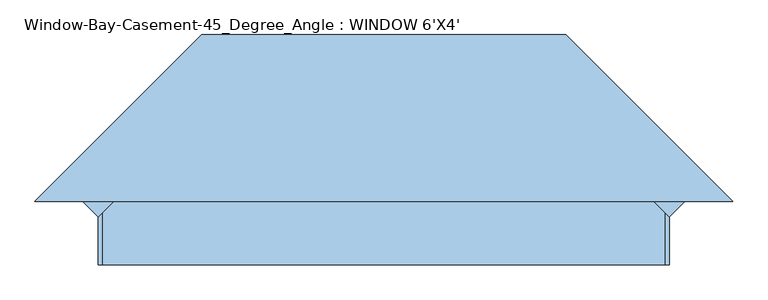
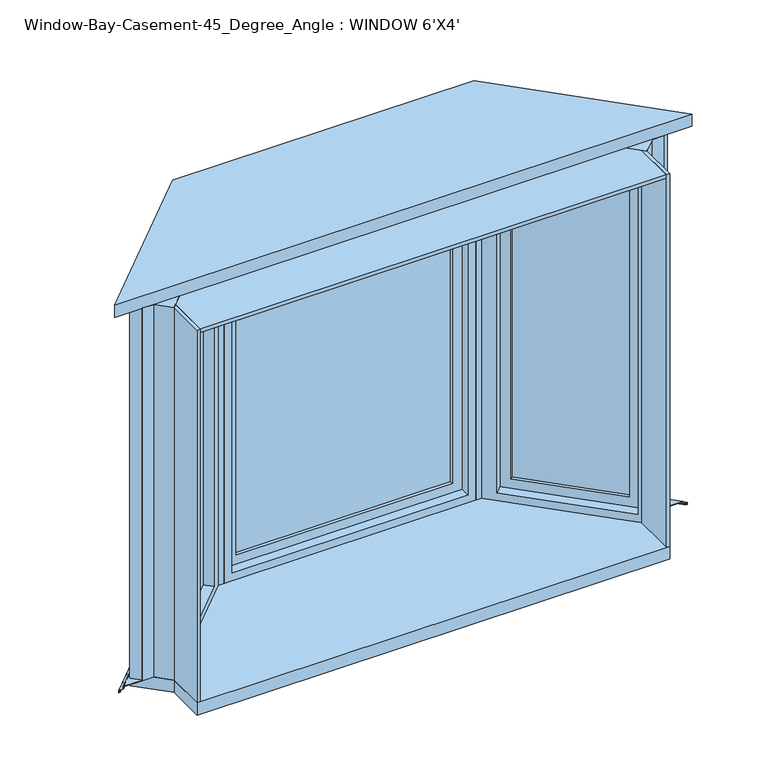
"""IFC4 building model written with IfcOpenShell, lengths in millimetres: window geometry, Window-Bay-Casement-45_Degree_Angle : WINDOW 6'X4'."""

from ifc_helpers import new_model, si_unit, frame, origin, place, context, project, spatial, polyline, outline, extrude, faceted_brep, source, transform, mapped, element, save


def window_bay_casement_45_degree_angle_window_6_x4_737bffb6(model_context):
    return source(origin(), model_context, "Body", "SolidModel", [
        extrude(outline(polyline([(914.4, 150.9914087), (909.9098719, 146.5012806), (619.1637138, 437.2474388), (623.6538418, 441.7375668), (914.4, 150.9914087)])), frame((0.0, 0.0, 730.25), z_axis=(0.0, 0.0, 1.0), x_axis=(1.0, 0.0, 0.0)), (0.0, 0.0, 1.0), 1384.3),
        extrude(outline(polyline([(905.4197439, 142.0111525), (900.9296158, 137.5210245), (610.1834576, 428.2671827), (614.6735857, 432.7573107), (905.4197439, 142.0111525)])), frame((0.0, 0.0, 730.25), z_axis=(0.0, 0.0, 1.0), x_axis=(1.0, 0.0, 0.0)), (0.0, 0.0, 1.0), 1384.3),
        extrude(outline(polyline([(1441.45, 57.15), (1441.45, -468.3271601), (-57.15, -468.3271601), (-57.15, 57.15), (1441.45, 57.15)]), holes=[polyline([(1384.3, -411.1771601), (1384.3, 0.0), (0.0, 0.0), (0.0, -411.1771601), (1384.3, -411.1771601)])]), frame((891.9493597, 128.5407684, 730.25), z_axis=(0.7071067811865468, 0.7071067811865483, 0.0), x_axis=(0.0, 0.0, 1.0)), (0.0, 0.0, 1.0), 44.45),
        faceted_brep([(509.4085913, 457.2, 2184.4), (914.4, 52.2085913, 2184.4), (963.7914087, 101.6, 2184.4), (1008.6926893, 101.6, 2184.4), (551.4926893, 558.8, 2184.4), (932.3605122, 88.1296158, 2171.7), (560.792049, 459.6980791, 2171.7), (605.6933296, 504.5993597, 2171.7), (977.2617928, 133.0308964, 2171.7), (891.9493597, 74.6592316, 2152.65), (547.3216648, 419.2869265, 2152.65), (574.2624332, 446.2276949, 2152.65), (918.8901281, 101.6, 2152.65), (560.792049, 459.6980791, 673.1), (605.6933296, 504.5993597, 673.1), (547.3216648, 419.2869265, 692.15), (574.2624332, 446.2276949, 692.15), (551.4926893, 558.8, 660.4), (1008.6926893, 101.6, 660.4), (963.7914087, 101.6, 660.4), (914.4, 52.2085913, 660.4), (509.4085913, 457.2, 660.4), (932.3605122, 88.1296158, 673.1), (977.2617928, 133.0308964, 673.1), (891.9493597, 74.6592316, 692.15), (918.8901281, 101.6, 692.15)], [[[0, 1, 2, 3, 4]], [[5, 6, 7, 8]], [[9, 10, 11, 12]], [[6, 13, 14, 7]], [[10, 15, 16, 11]], [[17, 18, 19, 20, 21]], [[13, 22, 23, 14]], [[15, 24, 25, 16]], [[20, 19, 2, 1]], [[3, 18, 17, 4], [7, 14, 23, 8]], [[8, 23, 22, 5]], [[5, 22, 13, 6], [11, 16, 25, 12]], [[12, 25, 24, 9]], [[1, 0, 21, 20], [9, 24, 15, 10]], [[4, 17, 21, 0]], [[2, 19, 18, 3]]]),
        extrude(outline(polyline([(-914.4, 150.9914087), (-623.6538418, 441.7375668), (-619.1637138, 437.2474388), (-909.9098719, 146.5012806), (-914.4, 150.9914087)])), frame((0.0, 0.0, 730.25), z_axis=(0.0, 0.0, 1.0), x_axis=(1.0, 0.0, 0.0)), (0.0, 0.0, 1.0), 1384.3),
        extrude(outline(polyline([(-905.4197439, 142.0111525), (-614.6735857, 432.7573107), (-610.1834576, 428.2671827), (-900.9296158, 137.5210245), (-905.4197439, 142.0111525)])), frame((0.0, 0.0, 730.25), z_axis=(0.0, 0.0, 1.0), x_axis=(1.0, 0.0, 0.0)), (0.0, 0.0, 1.0), 1384.3),
        extrude(outline(polyline([(1441.45, -57.15), (-57.15, -57.15), (-57.15, 468.3271601), (1441.45, 468.3271601), (1441.45, -57.15)]), holes=[polyline([(1384.3, 411.1771601), (0.0, 411.1771601), (0.0, 0.0), (1384.3, 0.0), (1384.3, 411.1771601)])]), frame((-891.9493597, 128.5407684, 730.25), z_axis=(-0.7071067811865468, 0.7071067811865483, 0.0), x_axis=(0.0, 0.0, 1.0)), (0.0, 0.0, 1.0), 44.45),
        faceted_brep([(-509.4085913, 457.2, 2184.4), (-551.4926893, 558.8, 2184.4), (-1008.6926893, 101.6, 2184.4), (-963.7914087, 101.6, 2184.4), (-914.4, 52.2085913, 2184.4), (-932.3605122, 88.1296158, 2171.7), (-977.2617928, 133.0308964, 2171.7), (-605.6933296, 504.5993597, 2171.7), (-560.792049, 459.6980791, 2171.7), (-891.9493597, 74.6592316, 2152.65), (-918.8901281, 101.6, 2152.65), (-574.2624332, 446.2276949, 2152.65), (-547.3216648, 419.2869265, 2152.65), (-605.6933296, 504.5993597, 673.1), (-560.792049, 459.6980791, 673.1), (-574.2624332, 446.2276949, 692.15), (-547.3216648, 419.2869265, 692.15), (-551.4926893, 558.8, 660.4), (-509.4085913, 457.2, 660.4), (-914.4, 52.2085913, 660.4), (-963.7914087, 101.6, 660.4), (-1008.6926893, 101.6, 660.4), (-977.2617928, 133.0308964, 673.1), (-932.3605122, 88.1296158, 673.1), (-918.8901281, 101.6, 692.15), (-891.9493597, 74.6592316, 692.15)], [[[0, 1, 2, 3, 4]], [[5, 6, 7, 8]], [[9, 10, 11, 12]], [[8, 7, 13, 14]], [[12, 11, 15, 16]], [[17, 18, 19, 20, 21]], [[14, 13, 22, 23]], [[16, 15, 24, 25]], [[19, 4, 3, 20]], [[2, 1, 17, 21], [7, 6, 22, 13]], [[6, 5, 23, 22]], [[5, 8, 14, 23], [11, 10, 24, 15]], [[10, 9, 25, 24]], [[4, 19, 18, 0], [9, 12, 16, 25]], [[1, 0, 18, 17]], [[3, 2, 21, 20]]]),
        faceted_brep([(-572.5347382, 609.6, 660.4), (-572.5347382, 609.6, 653.0697935), (572.5347382, 609.6, 653.0697935), (572.5347382, 609.6, 660.4), (-551.4926893, 558.8, 663.1486341), (-551.4926893, 558.8, 660.4), (551.4926893, 558.8, 660.4), (551.4926893, 558.8, 663.1486341), (-573.1133946, 610.997, 654.4483503), (-573.1133946, 610.997, 663.1486341), (573.1133946, 610.997, 663.1486341), (573.1133946, 610.997, 654.4483503), (578.3739068, 623.697, 652.2089977), (-578.3739068, 623.697, 652.2089977), (578.3739068, 623.697, 643.2668038), (-578.3739068, 623.697, 643.2668038), (-576.732627, 619.7346, 644.7270038), (-576.732627, 619.7346, 643.2668038), (576.732627, 619.7346, 643.2668038), (576.732627, 619.7346, 644.7270038), (-577.7110823, 622.0968, 650.8662705), (-577.7110823, 622.0968, 644.7270038), (577.7110823, 622.0968, 644.7270038), (577.7110823, 622.0968, 650.8662705), (-1080.5347382, 101.6, 660.4), (-1080.5347382, 101.6, 653.0697935), (1080.5347382, 101.6, 660.4), (1008.6926893, 101.6, 660.4), (-1008.6926893, 101.6, 660.4), (-1008.6926893, 101.6, 663.1486341), (1008.6926893, 101.6, 663.1486341), (1082.5103945, 101.6, 663.1486341), (-1082.5103945, 101.6, 663.1486341), (-1082.5103945, 101.6, 654.4483503), (-1100.4709068, 101.6, 652.2089977), (-1100.4709068, 101.6, 643.2668038), (1100.4709068, 101.6, 643.2668038), (1094.8672271, 101.6, 643.2668038), (-1094.8672271, 101.6, 643.2668038), (-1094.8672271, 101.6, 644.7270038), (1094.8672271, 101.6, 644.7270038), (1098.2078823, 101.6, 644.7270038), (-1098.2078823, 101.6, 644.7270038), (-1098.2078823, 101.6, 650.8662705), (1080.5347382, 101.6, 653.0697935), (1082.5103945, 101.6, 654.4483503), (1100.4709068, 101.6, 652.2089977), (1098.2078823, 101.6, 650.8662705)], [[[0, 1, 2, 3]], [[4, 5, 6, 7]], [[8, 9, 10, 11]], [[8, 11, 12, 13]], [[13, 12, 14, 15]], [[16, 17, 18, 19]], [[20, 21, 22, 23]], [[2, 1, 20, 23]], [[1, 0, 24, 25]], [[0, 3, 26, 27, 6, 5, 28, 24]], [[5, 4, 29, 28]], [[4, 7, 30, 31, 10, 9, 32, 29]], [[9, 8, 33, 32]], [[8, 13, 34, 33]], [[13, 15, 35, 34]], [[15, 14, 36, 37, 18, 17, 38, 35]], [[17, 16, 39, 38]], [[16, 19, 40, 41, 22, 21, 42, 39]], [[21, 20, 43, 42]], [[20, 1, 25, 43]], [[3, 2, 44, 26]], [[7, 6, 27, 30]], [[11, 10, 31, 45]], [[12, 11, 45, 46]], [[14, 12, 46, 36]], [[19, 18, 37, 40]], [[23, 22, 41, 47]], [[2, 23, 47, 44]], [[25, 24, 28, 29, 32, 33, 34, 35, 38, 39, 42, 43]], [[27, 26, 44, 47, 41, 40, 37, 36, 46, 45, 31, 30]]]),
        extrude(outline(polyline([(-986.242049, 124.0506403), (-1008.6926893, 101.6), (-1040.1235857, 133.0308964), (-1017.6729454, 155.4815367), (-986.242049, 124.0506403)])), frame((0.0, 0.0, 663.1486341), z_axis=(0.0, 0.0, 1.0), x_axis=(1.0, 0.0, 0.0)), (0.0, 0.0, 1.0), 1521.2513659),
        extrude(outline(polyline([(986.242049, 124.0506403), (1017.6729454, 155.4815367), (1040.1235857, 133.0308964), (1008.6926893, 101.6), (986.242049, 124.0506403)])), frame((0.0, 0.0, 663.1486341), z_axis=(0.0, 0.0, 1.0), x_axis=(1.0, 0.0, 0.0)), (0.0, 0.0, 1.0), 1521.2513659),
        extrude(outline(polyline([(583.0557627, 635.0), (1116.4557627, 101.6), (-1116.4557627, 101.6), (-583.0557627, 635.0), (583.0557627, 635.0)])), frame((0.0, 0.0, 2184.4), z_axis=(0.0, 0.0, 1.0), x_axis=(1.0, 0.0, 0.0)), (0.0, 0.0, 1.0), 50.8),
        extrude(outline(polyline([(-487.5414087, 558.8), (-487.5414087, 457.2), (-509.4085913, 457.2), (-551.4926893, 558.8), (-487.5414087, 558.8)])), frame((0.0, 0.0, 660.4), z_axis=(0.0, 0.0, 1.0), x_axis=(1.0, 0.0, 0.0)), (0.0, 0.0, 1.0), 1524.0),
        extrude(outline(polyline([(551.4926893, 558.8), (509.4085913, 457.2), (487.5414087, 457.2), (487.5414087, 558.8), (551.4926893, 558.8)])), frame((0.0, 0.0, 660.4), z_axis=(0.0, 0.0, 1.0), x_axis=(1.0, 0.0, 0.0)), (0.0, 0.0, 1.0), 1524.0),
        faceted_brep([(474.8414087, 495.3, 673.1), (474.8414087, 558.8, 673.1), (-474.8414087, 558.8, 673.1), (-474.8414087, 495.3, 673.1), (455.7914087, 457.2, 692.15), (455.7914087, 495.3, 692.15), (-455.7914087, 495.3, 692.15), (-455.7914087, 457.2, 692.15), (487.5414087, 558.8, 660.4), (487.5414087, 457.2, 660.4), (-487.5414087, 457.2, 660.4), (-487.5414087, 558.8, 660.4), (-474.8414087, 558.8, 2171.7), (-474.8414087, 495.3, 2171.7), (-455.7914087, 495.3, 2152.65), (-455.7914087, 457.2, 2152.65), (-487.5414087, 457.2, 2184.4), (-487.5414087, 558.8, 2184.4), (474.8414087, 558.8, 2171.7), (474.8414087, 495.3, 2171.7), (455.7914087, 495.3, 2152.65), (455.7914087, 457.2, 2152.65), (487.5414087, 457.2, 2184.4), (487.5414087, 558.8, 2184.4)], [[[0, 1, 2, 3]], [[4, 5, 6, 7]], [[8, 9, 10, 11]], [[3, 2, 12, 13]], [[7, 6, 14, 15]], [[11, 10, 16, 17]], [[13, 12, 18, 19]], [[15, 14, 20, 21]], [[17, 16, 22, 23]], [[11, 17, 23, 8], [1, 18, 12, 2]], [[19, 18, 1, 0]], [[3, 13, 19, 0], [5, 20, 14, 6]], [[21, 20, 5, 4]], [[9, 22, 16, 10], [7, 15, 21, 4]], [[23, 22, 9, 8]]]),
        extrude(outline(polyline([(417.6914087, 527.05), (417.6914087, 520.7), (-417.6914087, 520.7), (-417.6914087, 527.05), (417.6914087, 527.05)])), frame((0.0, 0.0, 730.25), z_axis=(0.0, 0.0, 1.0), x_axis=(1.0, 0.0, 0.0)), (0.0, 0.0, 1.0), 1384.3),
        extrude(outline(polyline([(417.6914087, 514.35), (417.6914087, 508.0), (-417.6914087, 508.0), (-417.6914087, 514.35), (417.6914087, 514.35)])), frame((0.0, 0.0, 730.25), z_axis=(0.0, 0.0, 1.0), x_axis=(1.0, 0.0, 0.0)), (0.0, 0.0, 1.0), 1384.3),
        extrude(outline(polyline([(914.4, -101.6), (-914.4, -101.6), (-914.4, 52.2085913), (-1022.1630735, 159.9716648), (-572.5347382, 609.6), (572.5347382, 609.6), (1022.1630735, 159.9716648), (914.4, 52.2085913), (914.4, -101.6)])), frame((0.0, 0.0, 609.6), z_axis=(0.0, 0.0, 1.0), x_axis=(1.0, 0.0, 0.0)), (0.0, 0.0, 1.0), 50.8),
        extrude(outline(polyline([(2171.7, -474.8414087), (673.1, -474.8414087), (673.1, 474.8414087), (2171.7, 474.8414087), (2171.7, -474.8414087)]), holes=[polyline([(2114.55, 417.6914087), (730.25, 417.6914087), (730.25, -417.6914087), (2114.55, -417.6914087), (2114.55, 417.6914087)])]), frame((0.0, 495.3, 0.0), z_axis=(0.0, 1.0, 0.0), x_axis=(0.0, 0.0, 1.0)), (0.0, 0.0, 1.0), 44.45),
        extrude(outline(polyline([(-914.4, -101.6), (-914.4, 52.2085913), (-901.7, 64.9085913), (-901.7, -101.6), (-914.4, -101.6)])), frame((0.0, 0.0, 660.4), z_axis=(0.0, 0.0, 1.0), x_axis=(1.0, 0.0, 0.0)), (0.0, 0.0, 1.0), 1524.0),
        extrude(outline(polyline([(914.4, -101.6), (901.7, -101.6), (901.7, 64.9085913), (914.4, 52.2085913), (914.4, -101.6)])), frame((0.0, 0.0, 660.4), z_axis=(0.0, 0.0, 1.0), x_axis=(1.0, 0.0, 0.0)), (0.0, 0.0, 1.0), 1524.0),
        extrude(outline(polyline([(-509.4085913, 457.2), (509.4085913, 457.2), (901.7, 64.9085913), (901.7, -101.6), (-901.7, -101.6), (-901.7, 64.9085913), (-509.4085913, 457.2)])), frame((0.0, 0.0, 2171.7), z_axis=(0.0, 0.0, 1.0), x_axis=(1.0, 0.0, 0.0)), (0.0, 0.0, 1.0), 12.7),
    ])


if __name__ == "__main__":
    model = new_model("IFC4")
    model_context = context("Model", 3, world=origin())
    ifc_project = project(units=[si_unit("LENGTHUNIT", "METRE", prefix="MILLI")], contexts=[model_context])
    site = spatial("IfcSite", under=ifc_project)
    building = spatial("IfcBuilding", under=site)
    placement = place(None, origin())
    window_bay_casement_45_degree_angle_window_6_x4_shape = window_bay_casement_45_degree_angle_window_6_x4_737bffb6(model_context)
    element("IfcWindow", 1, ObjectType="Window-Bay-Casement-45_Degree_Angle : WINDOW 6'X4'", at=placement, inside=building, context=model_context, shape_type="MappedRepresentation", body=[
        mapped(window_bay_casement_45_degree_angle_window_6_x4_shape, transform((0.0, 0.0, 0.0), x_axis=(1.0, 0.0, 0.0), y_axis=(0.0, 1.0, 0.0), z_axis=(0.0, 0.0, 1.0))),
    ])
    save(model, "model.ifc")

# Revit data of these elements
# Type "Window-Bay-Casement-45_Degree_Angle : WINDOW 6'X4'"
#   Type Mark = "20"
#   Fire Rating = "0.5h"
#   Assembly Code = "B2020100"
#   Analytic Construction = "Double glazing - domestic"
#   Width of Middle Sash = 3' - 2.38909"
#   Width = 6' - 0"
#   Visual Light Transmittance = 0.81
#   Thermal Resistance (R) = 1.8146 (h·ft²·°F)/BTU
#   Solar Heat Gain Coefficient = 0.76
#   Rough Width = 6' - 0 1/2"
#   Rough Height = 5' - 0 1/2"
#   Length 4 = 0' - 1.13909"
#   Length 3 = 0' - 0.51777"
#   Length 2 = 3' - 7.42462"
#   Length 1 = 1' - 2.80546"
#   Wall Thickness [instance default] = 0' - 6"
#   Trim Width = 6' - 5.03553"
#   Trim Height = 5' - 0"
#   Height 1 = 5' - 2"
#   Height = 5' - 0"
#   Heat Transfer Coefficient (U) = 0.5511 BTU/(h·ft²·°F)
#   Depth = 1' - 6"
#   Default Sill Height = 2' - 0"
#   Angle 1 = 22.50°
#   Angle = 45.00°
#   Center Muntin Visibility = yes
#   Side Muntin Visibility = yes
#   Interior Trim Visibility [instance default] = yes
#   Exterior Trim Visibility [instance default] = yes
#   Center Muntin Pattern = Muntin Pattern_2x2 : Muntin Pattern_2x2
#   Side Muntin Pattern = Muntin Pattern_2x2 : Muntin Pattern_2x2
#   Interior Trim Material = Wood - Stained
#   Exterior Trim Material = Clad - White
#   Exterior Trim = element 406231
#   Interior Trim = Trim-Window-Interior-Flat : Picture Frame
#   Interior Frame Material = Wood - Stained
#   Glass Panel Material = Glass
#   Exterior Frame Material = Clad - White
#   Wall Closure = (empty or 0)
# Element 1 (IfcWindow, "Window-Bay-Casement-45_Degree_Angle : WINDOW 6'X4'")
#   Wall Thickness = 0' - 8"
#   Materials on its faces: "Wood - Stained", "Clad - White", "Glass"
# Materials
#   "Wood - Stained": class "Wood", colour RGB 224 178 126, transparency 0, Cost = 0
#   "Clad - White": class "Wood", colour RGB 242 242 238, transparency 0, Cost = 0
#   "Glass": class "Glass", colour RGB 0 128 192, transparency 0.75, Description = "Soda Lime Glass", Cost = 0
